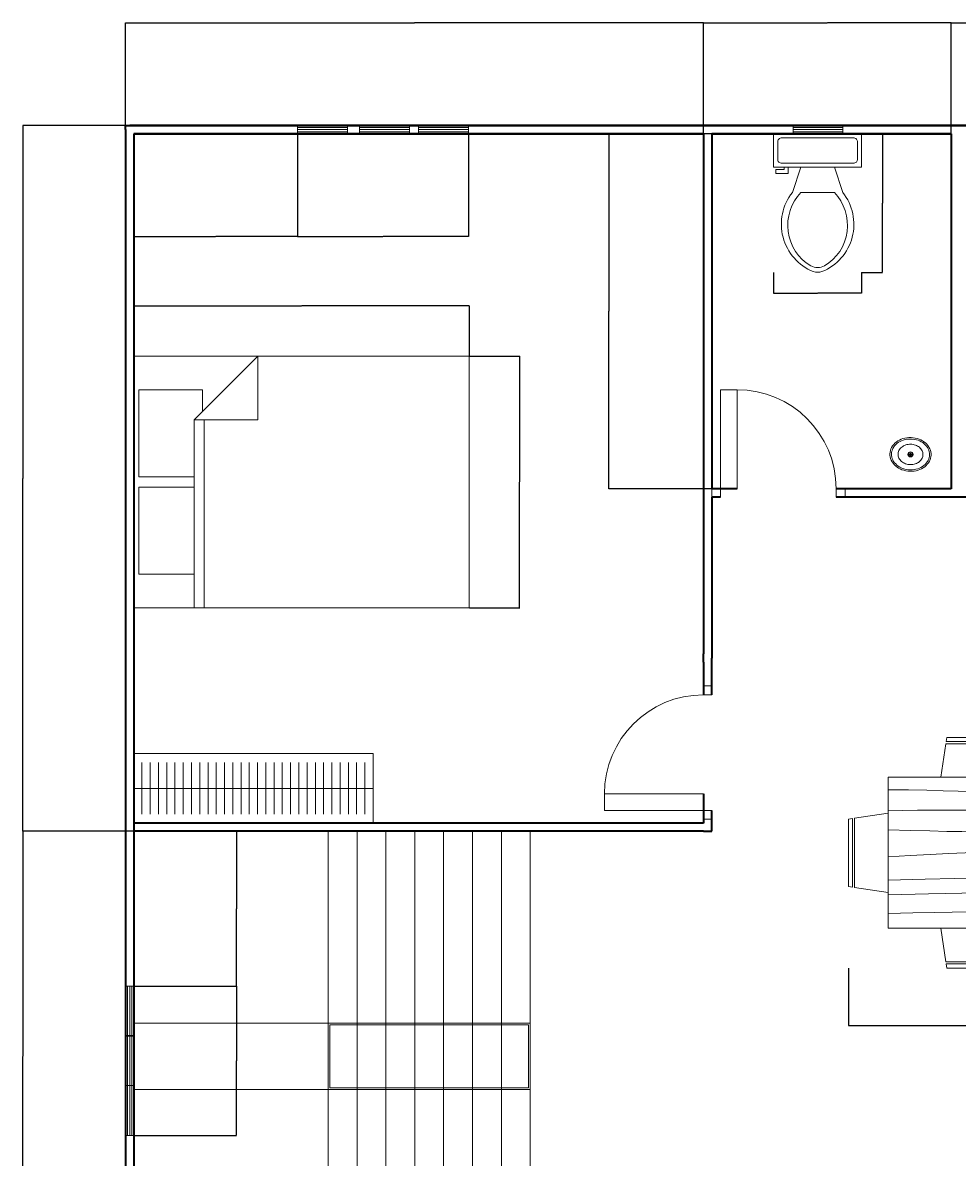
# Model space of a CAD drawing. Units: millimetres. Extents: x 1194 to 22780, y 83 to 13378.
# Tile 2 of 6: x 1194 to 6855, y 6507 to 13378. Entities that reach past the tile are written whole.
import ezdxf

# ---------------------------------------------------------------- set-up
doc = ezdxf.new("R2010")
doc.units = ezdxf.units.MM
for name, color, linetype, lineweight in [('A-ANNO-DIMS', 2, 'Continuous', 18), ('A-DOOR', 3, 'Continuous', 18), ('A-FLOR-CASE', 8, 'Continuous', 13), ('A-FLOR-FIXT', 9, 'Continuous', 18), ('A-FLOR-STRS', 7, 'Continuous', 18), ('A-FURN', 8, 'Continuous', 18), ('A-GLAZ', 4, 'Continuous', 18), ('A-WALL', 7, 'Continuous', 35)]:
    doc.layers.add(name, color=color, linetype=linetype, lineweight=lineweight)
doc.styles.get("Standard").update_dxf_attribs({"font": 'arial.ttf'})
doc.dimstyles.get("Standard").update_dxf_attribs({"dimtxt": 0.18, "dimasz": 0.18, "dimexe": 0.18, "dimexo": 0.0625, "dimgap": 0.09, "dimtad": 0, "dimtih": 1, "dimtoh": 1, "dimdec": 4, "dimzin": 0, "dimdsep": 46, "dimtxsty": 'Standard', "dimcen": 0.09, "dimadec": 0, "dimazin": 0, "dimtfac": 1, "dimtdec": 4, "dimtofl": 0, "dimtmove": 0, "dimatfit": 3, "dimfxl": 1, "dimtolj": 1, "dimtzin": 0, "dimarcsym": 0})

# ---------------------------------------------------------------- blocks, each defined once
blk = doc.blocks.new('Bed - Queen')
for p, q in [((0, -80.00003), (0, 0)), ((0, 0), (59.99999, 0)), ((59.99999, 0), (59.99999, -80.00003)), ((7.99999, -1.2), (28.79998, -1.2)), ((7.99999, -14.4), (7.99999, -1.2)), ((28.79998, -1.2), (28.79998, -14.4)), ((31.19999, -1.2), (51.99999, -1.2)), ((31.19999, -14.4), (31.19999, -1.2)), ((51.99999, -1.2), (51.99999, -16.4)), ((0, -14.4), (44.8, -14.4)), ((59.99999, -29.6), (44.8, -14.4)), ((44.8, -14.4), (44.8, -29.6)), ((44.8, -16.8), (0, -16.8)), ((51.99999, -16.4), (46.79936, -16.4)), ((44.8, -29.6), (59.99999, -29.6)), ((59.99999, -80.00003), (0, -80.00003))]:
    blk.add_line(p, q)
blk = doc.blocks.new('Dining Set - 36 x 72 in.')
for p, q in [((-22, 27.5), (-22.1562, 26.50042)), ((-22, 27.5), (-6, 27.5)), ((-5.8437, 26.49966), (-6, 27.5)), ((6, 27.5), (5.8438, 26.50042)), ((6, 27.5), (22, 27.5)), ((22.1563, 26.49966), (22, 27.5)), ((-22.2343, 26.00059), (-23.4847, 17.99762)), ((-22.2304, 26), (-5.7608, 26)), ((-5.8416, 26.5), (-22.1534, 26.5)), ((-4.5152, 17.99762), (-5.7655, 25.99926)), ((5.7657, 26.00059), (4.5153, 17.99762)), ((5.7696, 26), (22.2392, 26)), ((22.1584, 26.5), (5.8466, 26.5)), ((23.4848, 17.99762), (22.2345, 25.99926)), ((36, 18), (-36, 18)), ((-36, 18), (-36, -18)), ((36, -18), (36, 18)), ((-45.5, 8), (-44.5004, 8.15617)), ((-44.5, -8.15843), (-44.5, 8.15338)), ((-44.0006, 8.23428), (-35.9976, 9.48474)), ((-44, 8.23041), (-44, -8.23915)), ((44.0006, 8.23428), (35.9976, 9.48474)), ((44, 8.23041), (44, -8.23915)), ((44.5, -8.15843), (44.5, 8.15338)), ((45.5, 8), (44.5005, 8.15617)), ((-45.5, 8), (-45.5, -8)), ((45.5, 8), (45.5, -8)), ((-44.4997, -8.15631), (-45.5, -8)), ((44.4997, -8.15631), (45.5, -8)), ((-35.9976, -9.48476), (-43.9993, -8.2345)), ((35.9976, -9.48476), (43.9993, -8.2345)), ((-36, -18), (36, -18)), ((-22.2343, -26.0006), (-23.4847, -17.99762)), ((-4.5152, -17.99762), (-5.7655, -25.99928)), ((5.7657, -26.0006), (4.5153, -17.99762)), ((23.4848, -17.99762), (22.2345, -25.99928)), ((-22.2304, -26), (-5.7608, -26)), ((-22, -27.5), (-22.1562, -26.50044)), ((-5.8416, -26.5), (-22.1534, -26.5)), ((-5.8437, -26.49967), (-6, -27.5)), ((5.7696, -26), (22.2392, -26)), ((6, -27.5), (5.8438, -26.50044)), ((22.1584, -26.5), (5.8466, -26.5)), ((22.1563, -26.49967), (22, -27.5)), ((-22, -27.5), (-6, -27.5)), ((6, -27.5), (22, -27.5))]:
    blk.add_line(p, q)
for points in [[(-36, 15), (-31.1772, 14.97754), (-26.8079, 14.91406), (-22.8538, 14.81543), (-19.276, 14.6875), (-16.0362, 14.53613), (-13.0957, 14.36718), (-10.4159, 14.18652), (-7.9583, 14), (-5.6904, 13.81315), (-3.6035, 13.63021), (-1.6954, 13.45508), (0.0365, 13.29166), (1.5945, 13.14388), (2.9811, 13.01562), (4.1988, 12.9108), (5.25, 12.83333), (6.1393, 12.78613), (6.8802, 12.76823), (7.4883, 12.77767), (7.9792, 12.8125), (8.3685, 12.87077), (8.6719, 12.95052), (8.9049, 13.0498), (9.0833, 13.16666), (9.2205, 13.29899), (9.3216, 13.44401), (9.3895, 13.59879), (9.4271, 13.76041), (9.4373, 13.92594), (9.4232, 14.09245), (9.3875, 14.257), (9.3333, 14.41666), (9.2638, 14.56917), (9.1836, 14.71484), (9.0975, 14.85465), (9.0104, 14.98958), (8.9272, 15.1206), (8.8529, 15.2487), (8.7922, 15.37483), (8.75, 15.5), (8.7305, 15.62467), (8.7344, 15.74739), (8.7617, 15.86621), (8.8125, 15.97916), (8.8867, 16.08431), (8.9844, 16.17968), (9.1055, 16.26334), (9.25, 16.33333), (9.4189, 16.38802), (9.6172, 16.42708), (9.8506, 16.45052), (10.125, 16.45833), (10.4463, 16.45052), (10.8203, 16.42708), (11.2529, 16.38802), (11.75, 16.33333), (12.3184, 16.26318), (12.9694, 16.17838), (13.7151, 16.07991), (14.5677, 15.96875), (15.5395, 15.84586), (16.6426, 15.71224), (17.8893, 15.56884), (19.2917, 15.41666), (20.859, 15.25667), (22.5879, 15.08984), (24.4721, 14.91715), (26.5052, 14.73958), (28.6809, 14.5581), (30.9929, 14.3737), (33.4347, 14.18733), (36, 14)], [(-36, 10), (-28.9766, 10.14274), (-23.1725, 10.20442), (-18.4241, 10.19775), (-14.5677, 10.13541), (-11.4399, 10.03011), (-8.877, 9.89453), (-6.7154, 9.74137), (-4.7917, 9.58333), (-2.9698, 9.43082), (-1.2246, 9.28515), (0.4415, 9.14534), (2.026, 9.01041), (3.5266, 8.87939), (4.9408, 8.7513), (6.266, 8.62516), (7.5, 8.5), (8.6411, 8.37549), (9.6914, 8.2539), (10.6538, 8.13818), (11.5312, 8.03125), (12.3267, 7.93603), (13.043, 7.85547), (13.6831, 7.79248), (14.25, 7.75), (14.7471, 7.7303), (15.1797, 7.73307), (15.5537, 7.75732), (15.875, 7.80208), (16.1494, 7.86637), (16.3828, 7.94922), (16.5811, 8.04964), (16.75, 8.16666), (16.8944, 8.29915), (17.0143, 8.44531), (17.1089, 8.60319), (17.1771, 8.77083), (17.218, 8.94629), (17.2305, 9.1276), (17.2137, 9.31282), (17.1667, 9.5), (17.0895, 9.6875), (16.987, 9.875), (16.8649, 10.0625), (16.7292, 10.25), (16.5856, 10.4375), (16.4401, 10.625), (16.2985, 10.8125), (16.1667, 11), (16.05, 11.18733), (15.9518, 11.3737), (15.8752, 11.5581), (15.8229, 11.73958), (15.798, 11.91715), (15.8034, 12.08984), (15.842, 12.25667), (15.9167, 12.41666), (16.0295, 12.56836), (16.1784, 12.70833), (16.3605, 12.83268), (16.5729, 12.9375), (16.8127, 13.01888), (17.0768, 13.07291), (17.3625, 13.0957), (17.6667, 13.08333), (17.9894, 13.03312), (18.3418, 12.94726), (18.7382, 12.82918), (19.1927, 12.68229), (19.7195, 12.51001), (20.3327, 12.31575), (21.0465, 12.10294), (21.875, 11.875), (22.8357, 11.63354), (23.959, 11.37304), (25.2786, 11.08618), (26.8282, 10.76562), (28.6414, 10.40405), (30.752, 9.99414), (33.1936, 9.52856), (36, 9)], [(-36, 5.5), (-30.7157, 5.3348), (-26.069, 5.20963), (-21.9946, 5.11767), (-18.4271, 5.05208), (-15.3009, 5.00602), (-12.5508, 4.97265), (-10.1112, 4.94515), (-7.9167, 4.91666), (-5.909, 4.88167), (-4.0586, 4.83984), (-2.3429, 4.79215), (-0.7396, 4.73958), (0.7739, 4.6831), (2.22, 4.6237), (3.6213, 4.56233), (5, 4.5), (6.373, 4.43782), (7.7344, 4.3776), (9.0723, 4.32129), (10.375, 4.27083), (11.6309, 4.22819), (12.8281, 4.19531), (13.9551, 4.17415), (15, 4.16666), (15.954, 4.17448), (16.819, 4.19791), (17.6001, 4.23698), (18.3021, 4.29166), (18.9299, 4.36198), (19.4883, 4.44791), (19.9823, 4.54948), (20.4167, 4.66666), (20.7969, 4.79899), (21.1302, 4.94401), (21.4245, 5.09879), (21.6875, 5.26041), (21.9271, 5.42594), (22.1511, 5.59245), (22.3672, 5.757), (22.5834, 5.91666), (22.8065, 6.06868), (23.0404, 6.21093), (23.2879, 6.34147), (23.5521, 6.45833), (23.8358, 6.55957), (24.142, 6.64323), (24.4735, 6.70735), (24.8334, 6.75), (25.2235, 6.76969), (25.642, 6.76692), (26.0858, 6.74267), (26.5521, 6.69791), (27.0379, 6.63362), (27.5404, 6.55078), (28.0565, 6.45036), (28.5834, 6.33333), (29.1242, 6.19987), (29.7071, 6.04687), (30.3661, 5.87044), (31.1354, 5.66666), (32.0493, 5.43164), (33.142, 5.16146), (34.4475, 4.85221), (36, 4.5)], [(-36, -1), (-30.7915, -0.6591), (-26.0195, -0.38216), (-21.6519, -0.16284), (-17.6563, 0.00521), (-14.0005, 0.12833), (-10.6523, 0.21289), (-7.5796, 0.26522), (-4.75, 0.29166), (-2.134, 0.29793), (0.2878, 0.28711), (2.5317, 0.26163), (4.6146, 0.22396), (6.5529, 0.17651), (8.3633, 0.12174), (10.0623, 0.06209), (11.6667, 0), (13.1899, -0.06201), (14.6341, -0.1211), (15.9982, -0.17432), (17.2813, -0.21875), (18.4823, -0.25147), (19.6003, -0.26953), (20.6343, -0.27002), (21.5834, -0.25), (22.4481, -0.20768), (23.2357, -0.14584), (23.9549, -0.06836), (24.6146, 0.02083), (25.2235, 0.11784), (25.7904, 0.21875), (26.3241, 0.31966), (26.8334, 0.41666), (27.3265, 0.50618), (27.8099, 0.58593), (28.2894, 0.65397), (28.7709, 0.70833), (29.2601, 0.74707), (29.763, 0.76823), (30.2855, 0.76985), (30.8334, 0.75), (31.4088, 0.70784), (31.9994, 0.64713), (32.589, 0.57275), (33.1615, 0.48958), (33.7008, 0.4025), (34.1908, 0.3164), (34.6153, 0.23616), (34.9584, 0.16666), (35.2099, 0.11165), (35.3848, 0.07031), (35.504, 0.04069), (35.5886, 0.02083), (35.6594, 0.00879), (35.7377, 0.0026), (35.8442, 0.00032), (36, 0)], [(-36, -6.5), (-27.1843, -6.31267), (-20.084, -6.1263), (-14.469, -5.9419), (-10.1094, -5.76042), (-6.7752, -5.58285), (-4.2363, -5.41016), (-2.2629, -5.24333), (-0.625, -5.08334), (0.8708, -4.93099), (2.2715, -4.78646), (3.5872, -4.64974), (4.8281, -4.52084), (6.0046, -4.39974), (7.127, -4.28646), (8.2053, -4.18099), (9.25, -4.08334), (10.2705, -3.99382), (11.2734, -3.91407), (12.2647, -3.84603), (13.25, -3.79167), (14.2354, -3.75293), (15.2266, -3.73177), (16.2295, -3.73015), (17.25, -3.75), (18.2912, -3.79248), (19.3451, -3.85547), (20.4009, -3.93604), (21.4479, -4.03125), (22.4754, -4.13819), (23.4727, -4.25391), (24.4289, -4.37549), (25.3334, -4.5), (26.1785, -4.62492), (26.9694, -4.74935), (27.7145, -4.87281), (28.4219, -4.99479), (29.1, -5.11483), (29.7572, -5.23242), (30.4016, -5.34709), (31.0417, -5.45834), (31.6837, -5.56437), (32.3262, -5.65821), (32.9658, -5.73153), (33.599, -5.77604), (34.2224, -5.78345), (34.8327, -5.74545), (35.4264, -5.65373), (36, -5.5)], [(-36, -10), (-26.4022, -9.81299), (-18.4675, -9.62891), (-11.9839, -9.45069), (-6.7396, -9.28125), (-2.5226, -9.12354), (0.8789, -8.98047), (3.6769, -8.85498), (6.0833, -8.75), (8.2767, -8.66765), (10.3021, -8.60677), (12.1712, -8.56543), (13.8958, -8.54167), (15.4876, -8.53353), (16.9583, -8.53907), (18.3197, -8.55632), (19.5834, -8.58334), (20.7616, -8.61841), (21.8685, -8.66081), (22.9188, -8.71004), (23.9271, -8.76563), (24.9081, -8.82707), (25.8763, -8.89388), (26.8465, -8.96558), (27.8334, -9.04167), (28.8474, -9.12118), (29.8828, -9.20117), (30.93, -9.27824), (31.9792, -9.34896), (33.0205, -9.40991), (34.0443, -9.45768), (35.0407, -9.48885), (36, -9.5)], [(-36, -14.5), (-30.0881, -14.33513), (-25.0332, -14.21224), (-20.7312, -14.12647), (-17.0781, -14.07292), (-13.97, -14.04671), (-11.3027, -14.04297), (-8.9724, -14.05681), (-6.875, -14.08334), (-4.9224, -14.11833), (-3.0905, -14.16016), (-1.3709, -14.20785), (0.2448, -14.26042), (1.7647, -14.3169), (3.1973, -14.3763), (4.5507, -14.43767), (5.8333, -14.5), (7.0554, -14.5621), (8.235, -14.62175), (9.3922, -14.67652), (10.5469, -14.72396), (11.7192, -14.76164), (12.929, -14.78711), (14.1965, -14.79794), (15.5417, -14.79167), (16.9933, -14.76424), (18.6152, -14.70508), (20.4804, -14.60197), (22.6615, -14.44271), (25.2312, -14.21509), (28.2624, -13.9069), (31.8277, -13.50594), (36, -13)]]:
    blk.add_lwpolyline(points)
blk = doc.blocks.new('Sink - Oval top')
for p, q in [((-1, 0), (1, 0)), ((0, 1), (0, -1))]:
    blk.add_line(p, q)
for points in [[(-12.23, 0.39, 0.117634), (-11.46, -3.36, 0.104469), (-8.88, -6.8, 0.090016), (-5.08, -9.07, 0.08192), (-0.32, -10.02, 0.08192), (4.49, -9.38, 0.090016), (8.42, -7.36, 0.104469), (11.22, -4.09, 0.117634), (12.23, -0.39, 0.117634), (11.46, 3.36, 0.104469), (8.88, 6.8, 0.090016), (5.08, 9.07, 0.08192), (0.32, 10.02, 0.08192), (-4.49, 9.38, 0.090016), (-8.42, 7.36, 0.104469), (-11.22, 4.09, 0.117634)], [(-11.29, 0.16, 0.118622), (-10.52, -3.25, 0.104678), (-8.07, -6.36, 0.089562), (-4.54, -8.37, 0.081185), (-0.13, -9.15, 0.081185), (4.3, -8.49, 0.089562), (7.89, -6.58, 0.104678), (10.42, -3.55, 0.118622), (11.29, -0.16, 0.118622), (10.52, 3.25, 0.104678), (8.07, 6.36, 0.089562), (4.54, 8.37, 0.081185), (0.13, 9.15, 0.081185), (-4.3, 8.49, 0.089562), (-7.89, 6.58, 0.104678), (-10.42, 3.55, 0.118622)], [(-7.42, 0.08, 0.118283), (-6.91, -2.17, 0.104607), (-5.29, -4.21, 0.089718), (-2.97, -5.53, 0.081436), (-0.07, -6.04, 0.081436), (2.84, -5.59, 0.089718), (5.2, -4.33, 0.104607), (6.86, -2.32, 0.118283), (7.42, -0.08, 0.118283), (6.91, 2.17, 0.104607), (5.29, 4.21, 0.089718), (2.97, 5.53, 0.081436), (0.07, 6.04, 0.081436), (-2.84, 5.59, 0.089718), (-5.2, 4.33, 0.104607), (-6.86, 2.32, 0.118283)]]:
    blk.add_lwpolyline(points, format="xyb", close=True)
for radius in [1.5, 1]:
    blk.add_circle((0, 0), radius)
blk = doc.blocks.new('Toilet - top')
for p, q in [((9.5, -6), (9.5, -2)), ((-8, -8.5), (-8, -8)), ((-7, -8), (-7, -9.5)), ((-4, -8), (-6, -14)), ((4, -8), (6, -14)), ((-10, -8.5), (-8, -8.5)), ((-10, -9.5), (-10, -8.5)), ((-7, -9.5), (-10, -9.5)), ((4, -14), (-4, -14))]:
    blk.add_line(p, q)
blk.add_lwpolyline([(10.5, -8), (10.5, 0), (-10.5, 0), (-10.5, -8)], close=True)
for points in [[(-9.5, -2), (-9.5, -6)], [(8.5, -1), (-8.5, -1)], [(-8.5, -7), (8.5, -7)]]:
    blk.add_lwpolyline(points)
for centre, radius, start, end in [((-8.62, -1.88), 0.884, 81.8699, 188.1301), ((8.62, -1.88), 0.884, 351.8699, 98.1301), ((-8.62, -6.12), 0.884, 171.8699, 278.1301), ((8.62, -6.12), 0.884, 261.8699, 8.1301), ((3.52, -21.58), 12.17, 141.4691, 247.9714), ((4.2, -21.82), 11.33, 136.3677, 238.9468), ((-3.52, -21.58), 12.17, 292.0284, 38.5307), ((-4.2, -21.82), 11.33, 301.053, 43.6321), ((0, -27.88), 4, 245.7318, 294.2682), ((0, -29), 4, 254.8605, 285.1395)]:
    blk.add_arc(centre, radius, start, end)
blk = doc.blocks.new('Window - Wood Frame 36 in. Wide plan')
for p, q in [((0, 6), (0, 0)), ((0, 4.5), (36, 4.5)), ((0, 3), (36, 3)), ((0, 1.5), (36, 1.5)), ((36, 6), (36, 0))]:
    blk.add_line(p, q)
blk = doc.blocks.new('DOOR-SWING-600')
for p, q in [((0, 0), (0, 600)), ((0, 600), (100, 600)), ((100, 600), (100, 0))]:
    blk.add_line(p, q)
blk.add_arc((100, 0), 600, 0, 90)
blk = doc.blocks.new('STAIR-DUPLEX-FLIGHT')
for p, q in [((1177, 2725.9), (1177, 0)), ((1351.8, 2725.9), (1351.8, 0)), ((1526.7, 2725.9), (1526.7, 0)), ((1701.5, 2725.9), (1701.5, 0)), ((1876.4, 2725.9), (1876.4, 0)), ((2051.2, 2725.9), (2051.2, 0)), ((2226.1, 2725.9), (2226.1, 0)), ((2400.9, 2725.9), (2400.9, 0)), ((1177, 1562.9), (0, 1562.9)), ((2400.9, 1562.9), (1177, 1562.9)), ((1187, 1552.9), (2390.9, 1552.9)), ((1187, 1172.9), (1187, 1552.9)), ((2390.9, 1552.9), (2390.9, 1172.9)), ((2400.9, 1362.9), (2400.9, 1562.9)), ((2390.9, 1172.9), (1187, 1172.9)), ((2400.9, 1162.9), (0, 1162.9))]:
    blk.add_line(p, q)
blk = doc.blocks.new('WARDROBE-RAIL-1450')
for p, q in [((50, 156.2), (50, 312.4)), ((100, 156.2), (100, 312.4)), ((150, 156.2), (150, 312.4)), ((200, 156.2), (200, 312.4)), ((250, 156.2), (250, 312.4)), ((300, 156.2), (300, 312.4)), ((350, 156.2), (350, 312.4)), ((400, 156.2), (400, 312.4)), ((450, 156.2), (450, 312.4)), ((500, 156.2), (500, 312.4)), ((550, 156.2), (550, 312.4)), ((600, 156.2), (600, 312.4)), ((650, 156.2), (650, 312.4)), ((700, 156.2), (700, 312.4)), ((750, 156.2), (750, 312.4)), ((800, 156.2), (800, 312.4)), ((850, 156.2), (850, 312.4)), ((900, 156.2), (900, 312.4)), ((950, 156.2), (950, 312.4)), ((1000, 156.2), (1000, 312.4)), ((1050, 156.2), (1050, 312.4)), ((1100, 156.2), (1100, 312.4)), ((1150, 156.2), (1150, 312.4)), ((1200, 156.2), (1200, 312.4)), ((1250, 156.2), (1250, 312.4)), ((1300, 156.2), (1300, 312.4)), ((1350, 156.2), (1350, 312.4)), ((1400, 156.2), (1400, 312.4)), ((1450, 156.2), (1450, 312.4)), ((1450, 156.2), (0, 156.2)), ((50, 0), (50, 156.2)), ((100, 0), (100, 156.2)), ((150, 0), (150, 156.2)), ((200, 0), (200, 156.2)), ((250, 0), (250, 156.2)), ((300, 0), (300, 156.2)), ((350, 0), (350, 156.2)), ((400, 0), (400, 156.2)), ((450, 0), (450, 156.2)), ((500, 0), (500, 156.2)), ((550, 0), (550, 156.2)), ((600, 0), (600, 156.2)), ((650, 0), (650, 156.2)), ((700, 0), (700, 156.2)), ((750, 0), (750, 156.2)), ((800, 0), (800, 156.2)), ((850, 0), (850, 156.2)), ((900, 0), (900, 156.2)), ((950, 0), (950, 156.2)), ((1000, 0), (1000, 156.2)), ((1050, 0), (1050, 156.2)), ((1100, 0), (1100, 156.2)), ((1150, 0), (1150, 156.2)), ((1200, 0), (1200, 156.2)), ((1250, 0), (1250, 156.2)), ((1300, 0), (1300, 156.2)), ((1350, 0), (1350, 156.2)), ((1400, 0), (1400, 156.2))]:
    blk.add_line(p, q)
blk = doc.blocks.new('*D21')
at = {"layer": 'A-ANNO-DIMS', "color": 0, "lineweight": -2, "transparency": 16777216}
for p, q in [((1867.5, 11358.9), (1867.5, 11663.8)), ((1867.7, 11663.6), (2882.5, 11663.6)), ((3899.3, 11663.6), (2884.4, 11663.6)), ((3899.5, 11358.9), (3899.5, 11663.8))]:
    blk.add_line(p, q, dxfattribs=at)
at = {"layer": 'A-ANNO-DIMS', "color": 0, "transparency": 16777216}
for points in [[(1867.7, 11663.6), (1867.7, 11663.6), (1867.5, 11663.6)], [(3899.3, 11663.6), (3899.3, 11663.6), (3899.5, 11663.6)]]:
    blk.add_solid(points, dxfattribs=at)
at = {"layer": 'Defpoints', "color": 0, "transparency": 16777216}
for p in [(1867.5, 11663.6), (1867.5, 11358.8), (3899.5, 11358.8)]:
    blk.add_point(p, dxfattribs=at)
at = {"layer": 'A-ANNO-DIMS', "color": 0, "transparency": 16777216, "insert": (2883.5, 11663.6), "char_height": 0.18, "attachment_point": 5}
blk.add_mtext('\\A1;BED 2032 TYP.', dxfattribs=at)
blk = doc.blocks.new('*D22')
at = {"layer": 'A-ANNO-DIMS', "color": 0, "lineweight": -2, "transparency": 16777216}
for p, q in [((3899.5, 11358.8), (4204.5, 11358.8)), ((4204.3, 11358.6), (4204.3, 10597)), ((4204.3, 9835), (4204.3, 10596.6)), ((3899.5, 9834.8), (4204.5, 9834.8))]:
    blk.add_line(p, q, dxfattribs=at)
at = {"layer": 'A-ANNO-DIMS', "color": 0, "transparency": 16777216}
for points in [[(4204.3, 11358.6), (4204.3, 11358.6), (4204.3, 11358.8)], [(4204.3, 9835), (4204.3, 9835), (4204.3, 9834.8)]]:
    blk.add_solid(points, dxfattribs=at)
at = {"layer": 'Defpoints', "color": 0, "transparency": 16777216}
for p in [(3899.5, 11358.8), (4204.3, 11358.8), (3899.5, 9834.8)]:
    blk.add_point(p, dxfattribs=at)
at = {"layer": 'A-ANNO-DIMS', "color": 0, "transparency": 16777216, "insert": (4204.3, 10596.8), "char_height": 0.18, "attachment_point": 5}
blk.add_mtext('\\A1;1524 TYP.', dxfattribs=at)
blk = doc.blocks.new('*D27')
at = {"layer": 'A-ANNO-DIMS', "color": 0, "lineweight": -2, "transparency": 16777216}
for p, q in [((6275.6, 12705.8), (6401.6, 12705.8)), ((6401.4, 12705.6), (6401.4, 12286.3)), ((6401.4, 11866.6), (6401.4, 12285.9)), ((6275.6, 11866.4), (6401.6, 11866.4))]:
    blk.add_line(p, q, dxfattribs=at)
at = {"layer": 'A-ANNO-DIMS', "color": 0, "transparency": 16777216}
for points in [[(6401.4, 12705.6), (6401.5, 12705.6), (6401.4, 12705.8)], [(6401.4, 11866.6), (6401.5, 11866.6), (6401.4, 11866.4)]]:
    blk.add_solid(points, dxfattribs=at)
at = {"layer": 'Defpoints', "color": 0, "transparency": 16777216}
for p in [(6275.5, 12705.8), (6401.4, 12705.8), (6275.5, 11866.4)]:
    blk.add_point(p, dxfattribs=at)
at = {"layer": 'A-ANNO-DIMS', "color": 0, "transparency": 16777216, "insert": (6401.4, 12286.1), "char_height": 0.18, "attachment_point": 5}
blk.add_mtext('\\A1;WC 839 TYP.', dxfattribs=at)
blk = doc.blocks.new('*D28')
at = {"layer": 'A-ANNO-DIMS', "color": 0, "lineweight": -2, "transparency": 16777216}
for p, q in [((5742.1, 11866.3), (5742.1, 11740.3)), ((6275.5, 11866.3), (6275.5, 11740.3)), ((5742.3, 11740.5), (6008.2, 11740.5)), ((6275.3, 11740.5), (6009.4, 11740.5))]:
    blk.add_line(p, q, dxfattribs=at)
at = {"layer": 'A-ANNO-DIMS', "color": 0, "transparency": 16777216}
for points in [[(5742.3, 11740.5), (5742.3, 11740.5), (5742.1, 11740.5)], [(6275.3, 11740.5), (6275.3, 11740.5), (6275.5, 11740.5)]]:
    blk.add_solid(points, dxfattribs=at)
at = {"layer": 'Defpoints', "color": 0, "transparency": 16777216}
for p in [(5742.1, 11866.4), (6275.5, 11866.4), (6275.5, 11740.5)]:
    blk.add_point(p, dxfattribs=at)
at = {"layer": 'A-ANNO-DIMS', "color": 0, "transparency": 16777216, "insert": (6008.8, 11740.5), "char_height": 0.18, "attachment_point": 5}
blk.add_mtext('\\A1;533 TYP.', dxfattribs=at)
blk = doc.blocks.new('*D45')
at = {"layer": 'A-ANNO-DIMS', "color": 0, "lineweight": -2, "transparency": 16777216}
for p, q in [((6195, 7652.6), (6195, 7305.8)), ((8506.4, 7652.6), (8506.4, 7305.8)), ((6195.2, 7306), (7349.6, 7306)), ((8506.2, 7306), (7351.8, 7306))]:
    blk.add_line(p, q, dxfattribs=at)
at = {"layer": 'A-ANNO-DIMS', "color": 0, "transparency": 16777216}
for points in [[(6195.2, 7306), (6195.2, 7305.9), (6195, 7306)], [(8506.2, 7306), (8506.2, 7305.9), (8506.4, 7306)]]:
    blk.add_solid(points, dxfattribs=at)
at = {"layer": 'Defpoints', "color": 0, "transparency": 16777216}
for p in [(6195, 7652.7), (8506.4, 7652.7), (8506.4, 7306)]:
    blk.add_point(p, dxfattribs=at)
at = {"layer": 'A-ANNO-DIMS', "color": 0, "transparency": 16777216, "insert": (7350.7, 7306), "char_height": 0.18, "attachment_point": 5}
blk.add_mtext('\\A1;DINING SET 2311', dxfattribs=at)
blk = doc.blocks.new('*D53')
at = {"layer": 'A-ANNO-DIMS', "color": 0, "lineweight": -2, "transparency": 16777216}
for p, q in [((1817.5, 12755.8), (1817.5, 13378.5)), ((1817.7, 13378.3), (3567.1, 13378.3)), ((5317.3, 13378.3), (3567.8, 13378.3)), ((5317.5, 12705.8), (5317.5, 13378.5))]:
    blk.add_line(p, q, dxfattribs=at)
at = {"layer": 'A-ANNO-DIMS', "color": 0, "transparency": 16777216}
for points in [[(1817.7, 13378.3), (1817.7, 13378.2), (1817.5, 13378.3)], [(5317.3, 13378.3), (5317.3, 13378.2), (5317.5, 13378.3)]]:
    blk.add_solid(points, dxfattribs=at)
at = {"layer": 'Defpoints', "color": 0, "transparency": 16777216}
for p in [(5317.5, 13378.3), (1817.5, 12755.8), (5317.5, 12705.8)]:
    blk.add_point(p, dxfattribs=at)
at = {"layer": 'A-ANNO-DIMS', "color": 0, "transparency": 16777216, "insert": (3567.5, 13378.3), "char_height": 0.18, "attachment_point": 5}
blk.add_mtext('\\A1;3500', dxfattribs=at)
blk = doc.blocks.new('*D54')
at = {"layer": 'A-ANNO-DIMS', "color": 0, "lineweight": -2, "transparency": 16777216}
for p, q in [((5317.5, 12705.8), (5317.5, 13378.5)), ((5317.7, 13378.3), (6067.1, 13378.3)), ((6817.3, 13378.3), (6067.8, 13378.3)), ((6817.5, 12705.8), (6817.5, 13378.5))]:
    blk.add_line(p, q, dxfattribs=at)
at = {"layer": 'A-ANNO-DIMS', "color": 0, "transparency": 16777216}
for points in [[(5317.7, 13378.3), (5317.7, 13378.2), (5317.5, 13378.3)], [(6817.3, 13378.3), (6817.3, 13378.2), (6817.5, 13378.3)]]:
    blk.add_solid(points, dxfattribs=at)
at = {"layer": 'Defpoints', "color": 0, "transparency": 16777216}
for p in [(6817.5, 13378.3), (5317.5, 12705.8), (6817.5, 12705.8)]:
    blk.add_point(p, dxfattribs=at)
at = {"layer": 'A-ANNO-DIMS', "color": 0, "transparency": 16777216, "insert": (6067.5, 13378.3), "char_height": 0.18, "attachment_point": 5}
blk.add_mtext('\\A1;1500', dxfattribs=at)
blk = doc.blocks.new('*D55')
at = {"layer": 'A-ANNO-DIMS', "color": 0, "lineweight": -2, "transparency": 16777216}
for p, q in [((6817.5, 12705.8), (6817.5, 13378.5)), ((6817.7, 13378.3), (7567.1, 13378.3)), ((8317.3, 13378.3), (7567.8, 13378.3)), ((8317.5, 12705.8), (8317.5, 13378.5))]:
    blk.add_line(p, q, dxfattribs=at)
at = {"layer": 'A-ANNO-DIMS', "color": 0, "transparency": 16777216}
for points in [[(6817.7, 13378.3), (6817.7, 13378.2), (6817.5, 13378.3)], [(8317.3, 13378.3), (8317.3, 13378.2), (8317.5, 13378.3)]]:
    blk.add_solid(points, dxfattribs=at)
at = {"layer": 'Defpoints', "color": 0, "transparency": 16777216}
for p in [(8317.5, 13378.3), (6817.5, 12705.8), (8317.5, 12705.8)]:
    blk.add_point(p, dxfattribs=at)
at = {"layer": 'A-ANNO-DIMS', "color": 0, "transparency": 16777216, "insert": (7567.5, 13378.3), "char_height": 0.18, "attachment_point": 5}
blk.add_mtext('\\A1;1500', dxfattribs=at)
blk = doc.blocks.new('*D60')
at = {"layer": 'A-ANNO-DIMS', "color": 0, "lineweight": -2, "transparency": 16777216}
for p, q in [((1867.4, 8481.6), (1194.5, 8481.6)), ((1194.7, 8481.5), (1194.7, 7118.9)), ((1194.7, 5756), (1194.7, 7118.5)), ((1867.4, 5755.8), (1194.5, 5755.8))]:
    blk.add_line(p, q, dxfattribs=at)
at = {"layer": 'A-ANNO-DIMS', "color": 0, "transparency": 16777216}
for points in [[(1194.6, 8481.5), (1194.7, 8481.5), (1194.7, 8481.6)], [(1194.6, 5756), (1194.7, 5756), (1194.7, 5755.8)]]:
    blk.add_solid(points, dxfattribs=at)
at = {"layer": 'Defpoints', "color": 0, "transparency": 16777216}
for p in [(1194.7, 8481.6), (1867.5, 8481.6), (1867.5, 5755.8)]:
    blk.add_point(p, dxfattribs=at)
at = {"layer": 'A-ANNO-DIMS', "color": 0, "transparency": 16777216, "insert": (1194.7, 7118.7), "char_height": 0.18, "attachment_point": 5}
blk.add_mtext('\\A1;2726', dxfattribs=at)
blk = doc.blocks.new('*D61')
at = {"layer": 'A-ANNO-DIMS', "color": 0, "lineweight": -2, "transparency": 16777216}
for p, q in [((1817.4, 12755.8), (1194.5, 12755.8)), ((1194.7, 12755.6), (1194.7, 10618.9)), ((1194.7, 8481.8), (1194.7, 10618.5)), ((1867.4, 8481.6), (1194.5, 8481.6))]:
    blk.add_line(p, q, dxfattribs=at)
at = {"layer": 'A-ANNO-DIMS', "color": 0, "transparency": 16777216}
for points in [[(1194.6, 12755.6), (1194.7, 12755.6), (1194.7, 12755.8)], [(1194.6, 8481.8), (1194.7, 8481.8), (1194.7, 8481.6)]]:
    blk.add_solid(points, dxfattribs=at)
at = {"layer": 'Defpoints', "color": 0, "transparency": 16777216}
for p in [(1194.7, 12755.8), (1817.5, 12755.8), (1867.5, 8481.6)]:
    blk.add_point(p, dxfattribs=at)
at = {"layer": 'A-ANNO-DIMS', "color": 0, "transparency": 16777216, "insert": (1194.7, 10618.7), "char_height": 0.18, "attachment_point": 5}
blk.add_mtext('\\A1;4274', dxfattribs=at)
blk = doc.blocks.new('*D63')
at = {"layer": 'A-ANNO-DIMS', "color": 0, "lineweight": -2, "transparency": 16777216}
for p, q in [((5367.4, 12705.8), (4744.8, 12705.8)), ((4745, 12705.6), (4745, 11631)), ((4745, 10556), (4745, 11630.6)), ((5367.4, 10555.8), (4744.8, 10555.8))]:
    blk.add_line(p, q, dxfattribs=at)
at = {"layer": 'A-ANNO-DIMS', "color": 0, "transparency": 16777216}
for points in [[(4745, 12705.6), (4745, 12705.6), (4745, 12705.8)], [(4745, 10556), (4745, 10556), (4745, 10555.8)]]:
    blk.add_solid(points, dxfattribs=at)
at = {"layer": 'Defpoints', "color": 0, "transparency": 16777216}
for p in [(4745, 12705.8), (5367.5, 12705.8), (5367.5, 10555.8)]:
    blk.add_point(p, dxfattribs=at)
at = {"layer": 'A-ANNO-DIMS', "color": 0, "transparency": 16777216, "insert": (4745, 11630.8), "char_height": 0.18, "attachment_point": 5}
blk.add_mtext('\\A1;2150', dxfattribs=at)
blk = doc.blocks.new('*D65')
at = {"layer": 'A-ANNO-DIMS', "color": 0, "lineweight": -2, "transparency": 16777216}
for p, q in [((1867.5, 12705.7), (1867.3, 12083.1)), ((2859.3, 12705.4), (2859.1, 12082.8)), ((1867.5, 12083.3), (2362.8, 12083.1)), ((2858.9, 12082.9), (2363.6, 12083.1))]:
    blk.add_line(p, q, dxfattribs=at)
at = {"layer": 'A-ANNO-DIMS', "color": 0, "transparency": 16777216}
for points in [[(1867.5, 12083.3), (1867.5, 12083.2), (1867.3, 12083.3)], [(2858.9, 12083), (2858.9, 12082.9), (2859.1, 12082.9)]]:
    blk.add_solid(points, dxfattribs=at)
at = {"layer": 'Defpoints', "color": 0, "transparency": 16777216}
for p in [(1867.5, 12705.8), (2859.3, 12705.4), (1867.3, 12083.3)]:
    blk.add_point(p, dxfattribs=at)
at = {"layer": 'A-ANNO-DIMS', "color": 0, "transparency": 16777216, "insert": (2363.2, 12083.1), "char_height": 0.18, "attachment_point": 5}
blk.add_mtext('\\A1;991.9', dxfattribs=at)
blk = doc.blocks.new('*D66')
at = {"layer": 'A-ANNO-DIMS', "color": 0, "lineweight": -2, "transparency": 16777216}
for p, q in [((2859.3, 12705.4), (2859.3, 12082.8)), ((3894.4, 12705.4), (3894.4, 12082.8)), ((2859.5, 12082.9), (3376.5, 12082.9)), ((3894.3, 12082.9), (3377.3, 12082.9))]:
    blk.add_line(p, q, dxfattribs=at)
at = {"layer": 'A-ANNO-DIMS', "color": 0, "transparency": 16777216}
for points in [[(2859.5, 12083), (2859.5, 12082.9), (2859.3, 12082.9)], [(3894.3, 12083), (3894.3, 12082.9), (3894.4, 12082.9)]]:
    blk.add_solid(points, dxfattribs=at)
at = {"layer": 'Defpoints', "color": 0, "transparency": 16777216}
for p in [(2859.3, 12705.4), (3894.4, 12705.4), (2859.3, 12082.9)]:
    blk.add_point(p, dxfattribs=at)
at = {"layer": 'A-ANNO-DIMS', "color": 0, "transparency": 16777216, "insert": (3376.9, 12082.9), "char_height": 0.18, "attachment_point": 5}
blk.add_mtext('\\A1;1035.1', dxfattribs=at)
blk = doc.blocks.new('*D70')
at = {"layer": 'A-ANNO-DIMS', "color": 0, "lineweight": -2, "transparency": 16777216}
for p, q in [((1867.5, 7543.5), (2490.2, 7543.5)), ((2490, 7543.3), (2490, 7091.9)), ((2490, 6640.2), (2490, 7091.6)), ((1867.5, 6640), (2490.2, 6640))]:
    blk.add_line(p, q, dxfattribs=at)
at = {"layer": 'A-ANNO-DIMS', "color": 0, "transparency": 16777216}
for points in [[(2490, 7543.3), (2490, 7543.3), (2490, 7543.5)], [(2490, 6640.2), (2490, 6640.2), (2490, 6640)]]:
    blk.add_solid(points, dxfattribs=at)
at = {"layer": 'Defpoints', "color": 0, "transparency": 16777216}
for p in [(1867.5, 7543.5), (1867.5, 6640), (2490, 6640)]:
    blk.add_point(p, dxfattribs=at)
at = {"layer": 'A-ANNO-DIMS', "color": 0, "transparency": 16777216, "insert": (2490, 7091.7), "char_height": 0.18, "attachment_point": 5}
blk.add_mtext('\\A1;903.5', dxfattribs=at)
blk = doc.blocks.new('*D71')
at = {"layer": 'A-ANNO-DIMS', "color": 0, "lineweight": -2, "transparency": 16777216}
for p, q in [((1867.5, 8481.6), (2490.2, 8481.6)), ((2490, 8481.5), (2490, 8012.7)), ((2490, 7543.7), (2490, 8012.4)), ((1867.5, 7543.5), (2490.2, 7543.5))]:
    blk.add_line(p, q, dxfattribs=at)
at = {"layer": 'A-ANNO-DIMS', "color": 0, "transparency": 16777216}
for points in [[(2490, 8481.5), (2490, 8481.5), (2490, 8481.6)], [(2490, 7543.7), (2490, 7543.7), (2490, 7543.5)]]:
    blk.add_solid(points, dxfattribs=at)
at = {"layer": 'Defpoints', "color": 0, "transparency": 16777216}
for p in [(1867.5, 8481.6), (1867.5, 7543.5), (2490, 7543.5)]:
    blk.add_point(p, dxfattribs=at)
at = {"layer": 'A-ANNO-DIMS', "color": 0, "transparency": 16777216, "insert": (2490, 8012.6), "char_height": 0.18, "attachment_point": 5}
blk.add_mtext('\\A1;938.2', dxfattribs=at)

msp = doc.modelspace()

# ---------------------------------------------------------------- linework, layer by layer
at = {"layer": 'A-DOOR'}
for p, q in [((5367.481, 10555.774), (5367.481, 10505.774)), ((5421.166, 10505.774), (5421.166, 10555.774)), ((6121.166, 10555.774), (6121.166, 10505.774)), ((6174.851, 10505.774), (6174.851, 10555.774)), ((5367.481, 10505.774), (5421.166, 10505.774)), ((6121.166, 10505.774), (6174.851, 10505.774)), ((5367.481, 9361.492), (5317.481, 9361.492)), ((5317.481, 9307.807), (5317.481, 9361.492)), ((5367.481, 9307.807), (5367.481, 9361.492)), ((5317.481, 9307.807), (5367.481, 9307.807)), ((5317.481, 8554.123), (5317.481, 8707.807)), ((5367.481, 8607.807), (5317.481, 8607.807)), ((5367.481, 8554.123), (5367.481, 8607.807)), ((5317.481, 8554.123), (5367.481, 8554.123))]:
    msp.add_line(p, q, dxfattribs=at)
at = {"layer": 'A-FLOR-CASE'}
for p, q in [((1866.799, 8952.681), (1866.799, 8530.314)), ((3316.799, 8952.681), (1866.799, 8952.681)), ((3316.799, 8530.314), (3316.799, 8952.681)), ((1866.799, 8530.314), (3316.799, 8530.314))]:
    msp.add_line(p, q, dxfattribs=at)
at = {"layer": 'A-FLOR-STRS'}
for p, q in [((3044.45, 7318.705), (3044.45, 6918.705)), ((3044.45, 7318.705), (3044.45, 7308.705)), ((3044.45, 6918.705), (4268.39, 6918.705))]:
    msp.add_line(p, q, dxfattribs=at)
at = {"layer": 'A-WALL'}
for p, q in [((1817.481, 12730.774), (1817.481, 12755.774)), ((1817.481, 12755.774), (1842.481, 12755.774)), ((1817.481, 12730.774), (1817.481, 730.774)), ((10842.481, 12755.774), (1842.481, 12755.774)), ((1842.481, 12755.774), (5342.481, 12755.774)), ((1842.481, 12755.774), (10867.481, 12755.774)), ((5342.481, 12755.774), (6842.481, 12755.774)), ((1867.481, 12705.774), (1867.481, 9555.774)), ((1867.481, 12705.774), (5317.481, 12705.774)), ((5317.481, 12705.774), (1867.481, 12705.774)), ((5317.481, 12705.774), (5317.481, 9555.774)), ((5367.481, 12705.774), (5367.481, 10555.774)), ((5367.481, 12705.774), (6817.481, 12705.774)), ((6817.481, 12705.774), (5367.481, 12705.774)), ((6817.481, 12705.774), (6817.481, 10555.774)), ((5521.166, 10555.774), (5367.481, 10555.774)), ((6817.481, 10555.774), (6121.166, 10555.774)), ((5367.481, 10505.774), (5367.481, 9530.774)), ((5421.166, 10505.774), (5367.481, 10505.774)), ((6842.481, 10505.774), (6121.166, 10505.774)), ((6921.111, 10505.774), (6842.481, 10505.774)), ((1867.481, 9555.774), (1867.481, 9505.774)), ((5317.481, 9505.774), (5317.481, 9555.774)), ((1867.481, 9505.774), (1867.481, 5755.774)), ((5317.481, 9505.774), (5317.481, 9307.807)), ((5367.481, 9307.807), (5367.481, 9530.774)), ((5317.481, 8707.807), (5317.481, 8531.636)), ((5367.481, 8481.636), (5367.481, 8607.807)), ((5317.481, 8531.636), (1867.481, 8531.636)), ((5317.481, 8481.636), (1867.481, 8481.636)), ((5317.481, 8481.636), (5367.481, 8481.636))]:
    msp.add_line(p, q, dxfattribs=at)

# ---------------------------------------------------------------- block references
at = {"layer": 'A-DOOR'}
msp.add_blockref('DOOR-SWING-600', (5421.166, 10555.774), dxfattribs=at)
at = {"layer": 'A-DOOR', "rotation": 90.00000000000006}
msp.add_blockref('DOOR-SWING-600', (5317.481, 8607.808), dxfattribs=at)
at = {"layer": 'A-FLOR-CASE'}
msp.add_blockref('WARDROBE-RAIL-1450', (1866.799, 8585.292), dxfattribs=at)
at = {"layer": 'A-FLOR-FIXT'}
for name, p, xscale, yscale, zscale in [('Toilet - top', (6008.825, 12705.774), 25.4, 25.4, 25.4), ('Sink - Oval top', (6571.476, 10763.902), 10.19841034025665, 10.19841034025665, 10.19841034025665)]:
    msp.add_blockref(name, p, dxfattribs=dict(at, xscale=xscale, yscale=yscale, zscale=zscale))
at = {"layer": 'A-FLOR-STRS'}
msp.add_blockref('STAIR-DUPLEX-FLIGHT', (1867.481, 5755.774), dxfattribs=at)
at = {"layer": 'A-FURN', "xscale": 25.4, "yscale": 25.4, "zscale": 25.4, "rotation": 90}
msp.add_blockref('Bed - Queen', (1867.481, 9834.806), dxfattribs=at)
at = {"layer": 'A-FURN', "xscale": 25.4, "yscale": 25.4, "zscale": 25.4}
msp.add_blockref('Dining Set - 36 x 72 in.', (7350.673, 8351.169), dxfattribs=at)
at = {"layer": 'A-GLAZ', "xscale": 8.388003104210137, "yscale": 8.388003104210137, "zscale": 8.388003104210137}
for p in [(2859.334, 12705.446), (3234.324, 12705.446), (3592.481, 12705.446), (5860.438, 12705.446)]:
    msp.add_blockref('Window - Wood Frame 36 in. Wide plan', p, dxfattribs=at)
at = {"layer": 'A-GLAZ', "xscale": 8.388003104210137, "yscale": 8.388003104210137, "zscale": 8.388003104210137, "rotation": 90}
for p in [(1867.481, 7241.517), (1867.481, 6941.98), (1867.481, 6640.012)]:
    msp.add_blockref('Window - Wood Frame 36 in. Wide plan', p, dxfattribs=at)

# ---------------------------------------------------------------- dimensions: what is measured, and where the dimension line sits
at = {"layer": 'A-ANNO-DIMS'}
for base, p1, p2, picture, middle in [((5317.481, 13378.274), (1817.481, 12755.774), (5317.481, 12705.774), '*D53', (3567.481, 13378.274)), ((6817.481, 13378.274), (5317.481, 12705.774), (6817.481, 12705.774), '*D54', (6067.481, 13378.274)), ((8317.481, 13378.274), (6817.481, 12705.774), (8317.481, 12705.774), '*D55', (7567.481, 13378.274))]:
    dim = msp.add_linear_dim(base=base, p1=p1, p2=p2, dimstyle='Standard', override={"dimdec": 0, "dimlfac": 1, "dimrnd": 0, "dimzin": 0, "dimdsep": 46, "dimlunit": 2}, dxfattribs=at)
    dim.commit()
    dim.dimension.update_dxf_attribs({"geometry": picture, "text_midpoint": middle})
for base, p1, p2, angle, override, picture, middle in [((1194.653, 12755.774), (1867.481, 8481.636), (1817.481, 12755.774), 90, {"dimdec": 0, "dimlfac": 1, "dimrnd": 0, "dimzin": 0, "dimdsep": 46, "dimlunit": 2}, '*D61', (1194.653, 10618.705)), ((1867.275, 12083.274), (2859.334, 12705.446), (1867.481, 12705.774), 179.9810515, {"dimdec": 1, "dimlfac": 1, "dimrnd": 0, "dimzin": 0, "dimdsep": 46, "dimlunit": 2}, '*D65', (2363.201, 12083.11)), ((2859.334, 12082.946), (3894.449, 12705.446), (2859.334, 12705.446), 180, {"dimdec": 1, "dimlfac": 1, "dimrnd": 0, "dimzin": 0, "dimdsep": 46, "dimlunit": 2}, '*D66', (3376.891, 12082.946)), ((4744.981, 12705.774), (5367.481, 10555.774), (5367.481, 12705.774), 90, {"dimdec": 0, "dimlfac": 1, "dimrnd": 0, "dimzin": 0, "dimdsep": 46, "dimlunit": 2}, '*D63', (4744.981, 11630.774)), ((1194.653, 8481.636), (1867.481, 5755.774), (1867.481, 8481.636), 90, {"dimdec": 0, "dimlfac": 1, "dimrnd": 0, "dimzin": 0, "dimdsep": 46, "dimlunit": 2}, '*D60', (1194.653, 7118.705)), ((2489.981, 7543.485), (1867.481, 8481.636), (1867.481, 7543.485), 270, {"dimdec": 1, "dimlfac": 1, "dimrnd": 0, "dimzin": 0, "dimdsep": 46, "dimlunit": 2}, '*D71', (2489.981, 8012.561)), ((2489.981, 6640.012), (1867.481, 7543.485), (1867.481, 6640.012), 270, {"dimdec": 1, "dimlfac": 1, "dimrnd": 0, "dimzin": 0, "dimdsep": 46, "dimlunit": 2}, '*D70', (2489.981, 7091.748))]:
    dim = msp.add_linear_dim(base=base, p1=p1, p2=p2, angle=angle, dimstyle='Standard', override=override, dxfattribs=at)
    dim.commit()
    dim.dimension.update_dxf_attribs({"geometry": picture, "text_midpoint": middle})
for base, p1, p2, angle, text, picture, middle in [((6401.431, 12705.774), (6275.525, 11866.399), (6275.525, 12705.774), 90, 'WC <> TYP.', '*D27', (6401.431, 12286.087)), ((1867.481, 11663.606), (3899.482, 11358.806), (1867.481, 11358.806), 180, 'BED <> TYP.', '*D21', (2883.481, 11663.606)), ((4204.282, 11358.806), (3899.482, 9834.806), (3899.482, 11358.806), 90, '<> TYP.', '*D22', (4204.282, 10596.806))]:
    dim = msp.add_linear_dim(base=base, p1=p1, p2=p2, angle=angle, text=text, dimstyle='Standard', override={"dimdec": 0, "dimlfac": 1, "dimrnd": 0, "dimzin": 0, "dimdsep": 46, "dimlunit": 2}, dxfattribs=at)
    dim.commit()
    dim.dimension.update_dxf_attribs({"geometry": picture, "text_midpoint": middle})
for base, p1, p2, text, picture, middle in [((6275.525, 11740.493), (5742.125, 11866.399), (6275.525, 11866.399), '<> TYP.', '*D28', (6008.825, 11740.493)), ((8506.373, 7305.959), (6194.973, 7652.669), (8506.373, 7652.669), 'DINING SET <>', '*D45', (7350.673, 7305.959))]:
    dim = msp.add_linear_dim(base=base, p1=p1, p2=p2, text=text, dimstyle='Standard', override={"dimdec": 0, "dimlfac": 1, "dimrnd": 0, "dimzin": 0, "dimdsep": 46, "dimlunit": 2}, dxfattribs=at)
    dim.commit()
    dim.dimension.update_dxf_attribs({"geometry": picture, "text_midpoint": middle})

doc.saveas('drawing.dxf')
